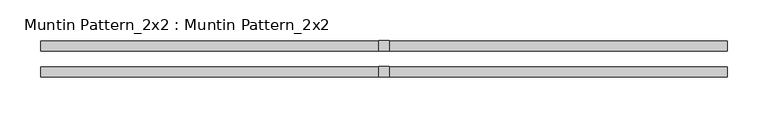
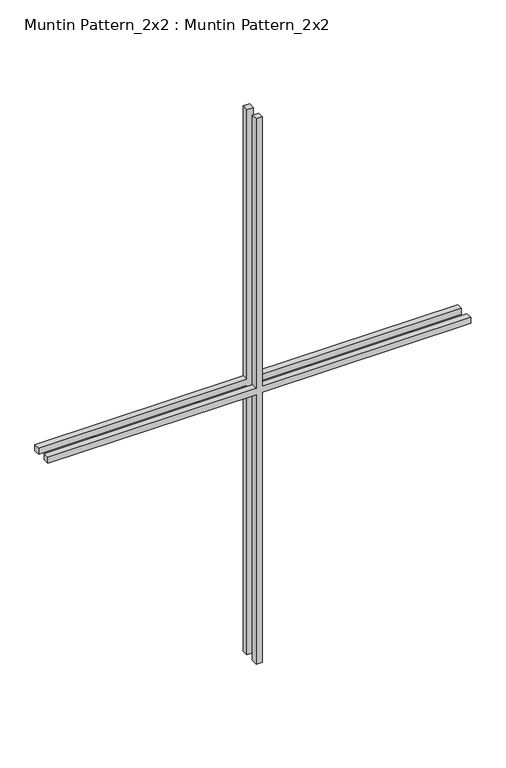
"""IFC4 building model written with IfcOpenShell, lengths in millimetres: proxy geometry, Muntin Pattern_2x2 : Muntin Pattern_2x2."""

from ifc_helpers import new_model, si_unit, frame, origin, place, context, project, spatial, polyline, outline, extrude, source, transform, mapped, element, save


def muntin_pattern_2x2_muntin_pattern_2x2_0b2f62cf(model_context):
    return source(origin(), model_context, "Body", "SweptSolid", [
        extrude(outline(polyline([(577.85, -6.35), (577.85, -419.1), (565.15, -419.1), (565.15, -6.35), (0.0, -6.35), (0.0, 6.35), (565.15, 6.35), (565.15, 419.1), (577.85, 419.1), (577.85, 6.35), (1143.0, 6.35), (1143.0, -6.35), (577.85, -6.35)])), frame((0.0, -22.225, 0.0), z_axis=(0.0, 1.0, 0.0), x_axis=(0.0, 0.0, 1.0)), (0.0, 0.0, 1.0), 12.7),
        extrude(outline(polyline([(577.85, -6.35), (577.85, -419.1), (565.15, -419.1), (565.15, -6.35), (0.0, -6.35), (0.0, 6.35), (565.15, 6.35), (565.15, 419.1), (577.85, 419.1), (577.85, 6.35), (1143.0, 6.35), (1143.0, -6.35), (577.85, -6.35)])), frame((0.0, 9.525, 0.0), z_axis=(0.0, 1.0, 0.0), x_axis=(0.0, 0.0, 1.0)), (0.0, 0.0, 1.0), 12.7),
    ])


if __name__ == "__main__":
    model = new_model("IFC4")
    model_context = context("Model", 3, world=origin())
    ifc_project = project(units=[si_unit("LENGTHUNIT", "METRE", prefix="MILLI")], contexts=[model_context])
    site = spatial("IfcSite", under=ifc_project)
    building = spatial("IfcBuilding", under=site)
    placement = place(None, origin())
    muntin_pattern_2x2_muntin_pattern_2x2_shape = muntin_pattern_2x2_muntin_pattern_2x2_0b2f62cf(model_context)
    element("IfcBuildingElementProxy", 1, Name="Muntin Pattern_2x2 : Muntin Pattern_2x2", ObjectType="Muntin Pattern_2x2 : Muntin Pattern_2x2", at=placement, inside=building, context=model_context, shape_type="MappedRepresentation", body=[
        mapped(muntin_pattern_2x2_muntin_pattern_2x2_shape, transform((0.0, 0.0, 0.0), x_axis=(1.0, 0.0, 0.0), y_axis=(0.0, 1.0, 0.0), z_axis=(0.0, 0.0, 1.0))),
    ])
    save(model, "model.ifc")

# Revit data of these elements
# Type "Muntin Pattern_2x2 : Muntin Pattern_2x2"
#   Width [instance default] = 4' - 0"
#   Thickness = 0' - 0 1/2"
#   Height [instance default] = 4' - 0"
#   Distance = 0' - 0 3/4"
#   Interior Material [instance default] = none
#   Exterior Material [instance default] = none
#   Default Elevation = 0
# Element 1 (IfcBuildingElementProxy, "Muntin Pattern_2x2 : Muntin Pattern_2x2")
#   Width = 2' - 9"
#   Height = 3' - 9"
#   Interior Material = Wood - Stained
#   Exterior Material = Clad - White
#   Materials on its faces: "Clad - White", "Wood - Stained"
# Materials
#   "Clad - White": class "Wood", colour RGB 245 245 243, transparency 0, Cost = 0
#   "Wood - Stained": class "Wood", colour RGB 173 132 96, transparency 0, Cost = 0
